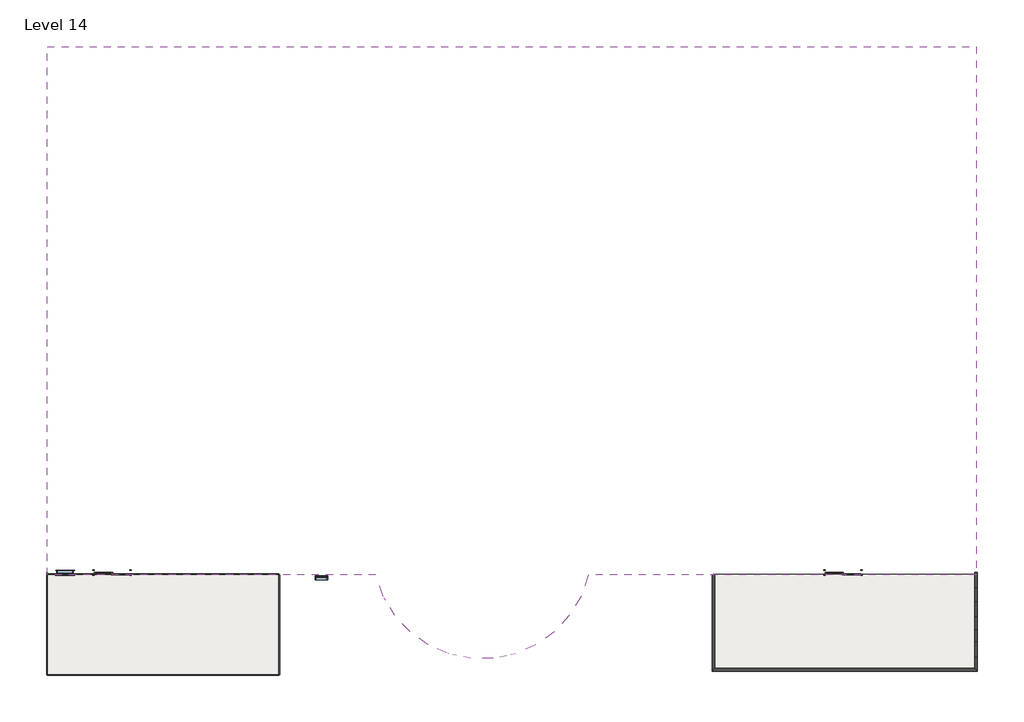
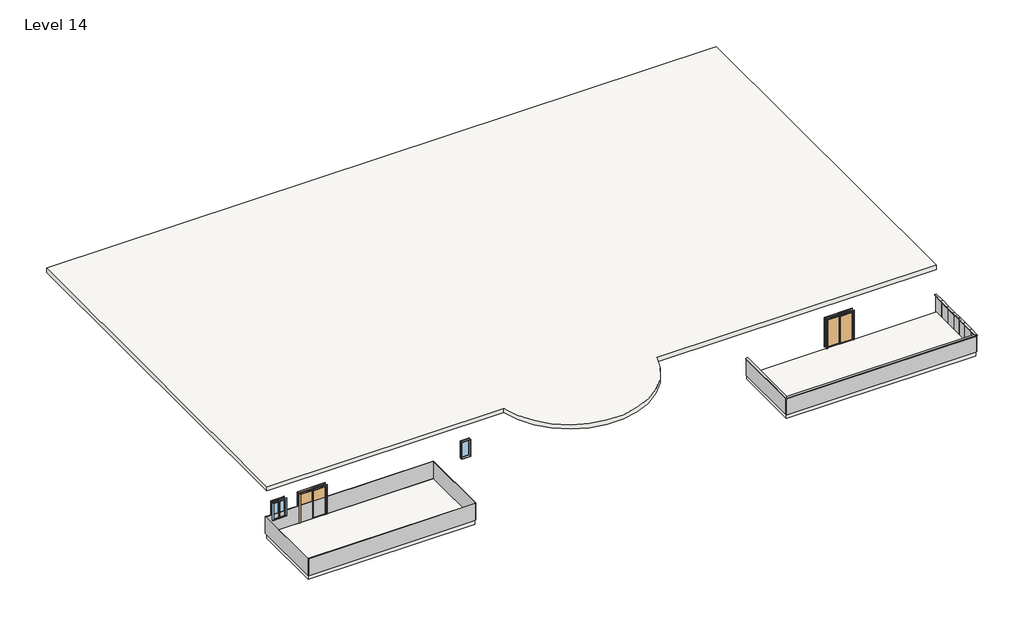
# One storey: 13 plates, 9 members, 3 slabs, 2 doors, 2 windows.
"""IFC4 building model written with IfcOpenShell, lengths in millimetres."""

from ifc_helpers import new_model, si_unit, point, frame, frame_2d, origin, place, context, project, spatial, polyline, circle_curve, trimmed, segment, composite_curve, outline, extrude, transform, mapped, element, save
from components import door_076b30e0, member_47bfaf8a, member_aa870034, member_0b2b3a95, member_df81370e, member_5882a209, member_d818a040, system_panel_glazed_f269d4c8, system_panel_glazed_7af1c9c3, system_panel_glazed_4f3cd66b, system_panel_glazed_7cd9bc56, system_panel_glazed_7fa16c81, system_panel_glazed_ea481271, system_panel_glazed_53c2349a, system_panel_glazed_dfd0d0b7, window_bb17773d, window_80bd9af0

model = new_model("IFC4")

# Units and contexts
model_context = context("Model", 3, world=origin())
ifc_project = project(units=[si_unit("LENGTHUNIT", "METRE", prefix="MILLI")], contexts=[model_context])

# Site, building, storey
site = spatial("IfcSite", under=ifc_project)
building = spatial("IfcBuilding", under=site)
storey = spatial("IfcBuildingStorey", under=building, Name="Level 14", Elevation=23164.8)

# Doors
placement = place(None, origin())
door_shape = door_076b30e0(model_context)
element("IfcDoor", 1, ObjectType="Door-Double-Sliding : 68\" x 80\"", at=placement, inside=storey, context=model_context, shape_type="MappedRepresentation", body=[
    mapped(door_shape, transform((-16674.185279, -12227.7237084, 23164.8), x_axis=(-1.0, 0.0, 0.0), y_axis=(0.0, -1.0, 0.0), z_axis=(0.0, 0.0, 1.0))),
])
element("IfcDoor", 2, ObjectType="Door-Double-Sliding : 68\" x 80\"", at=placement, inside=storey, context=model_context, shape_type="MappedRepresentation", body=[
    mapped(door_shape, transform((18987.414721, -12227.7237084, 23164.8), x_axis=(-1.0, 0.0, 0.0), y_axis=(0.0, -1.0, 0.0), z_axis=(0.0, 0.0, 1.0))),
])

# Members
member_shape = member_47bfaf8a(model_context)
element("IfcMember", 3, ObjectType="Rectangular Mullion : 2.5\" x 5\" rectangular", at=placement, inside=storey, context=model_context, shape_type="MappedRepresentation", body=[
    mapped(member_shape, transform((25489.814721, -15121.4141485, 24384.0), x_axis=(0.0, 0.0, 1.0), y_axis=(-1.0, 0.0, 0.0), z_axis=(0.0, -1.0, 0.0))),
])
element("IfcMember", 4, ObjectType="Rectangular Mullion : 2.5\" x 5\" rectangular", at=placement, inside=storey, context=model_context, shape_type="MappedRepresentation", body=[
    mapped(member_shape, transform((25489.814721, -15731.0141485, 24384.0), x_axis=(0.0, 0.0, 1.0), y_axis=(-1.0, 0.0, 0.0), z_axis=(0.0, -1.0, 0.0))),
])
member_2_shape = member_aa870034(model_context)
element("IfcMember", 5, ObjectType="Rectangular Mullion : 2.5\" x 5\" rectangular", at=placement, inside=storey, context=model_context, shape_type="MappedRepresentation", body=[
    mapped(member_2_shape, transform((25489.814721, -16493.0141485, 24384.0), x_axis=(0.0, 0.0, 1.0), y_axis=(-1.0, 0.0, 0.0), z_axis=(0.0, -1.0, 0.0))),
])
member_3_shape = member_0b2b3a95(model_context)
element("IfcMember", 6, ObjectType="Rectangular Mullion : 2.5\" x 5\" rectangular", at=placement, inside=storey, context=model_context, shape_type="MappedRepresentation", body=[
    mapped(member_3_shape, transform((25489.814721, -13073.7538551, 24384.0), x_axis=(0.0, 0.0, 1.0), y_axis=(-1.0, 0.0, 0.0), z_axis=(0.0, -1.0, 0.0))),
])
element("IfcMember", 7, ObjectType="Rectangular Mullion : 2.5\" x 5\" rectangular", at=placement, inside=storey, context=model_context, shape_type="MappedRepresentation", body=[
    mapped(member_3_shape, transform((25489.814721, -13792.7840018, 24384.0), x_axis=(0.0, 0.0, 1.0), y_axis=(-1.0, 0.0, 0.0), z_axis=(0.0, -1.0, 0.0))),
])
element("IfcMember", 8, ObjectType="Rectangular Mullion : 2.5\" x 5\" rectangular", at=placement, inside=storey, context=model_context, shape_type="MappedRepresentation", body=[
    mapped(member_3_shape, transform((25489.814721, -14511.8141485, 24384.0), x_axis=(0.0, 0.0, 1.0), y_axis=(-1.0, 0.0, 0.0), z_axis=(0.0, -1.0, 0.0))),
])
member_4_shape = member_df81370e(model_context)
element("IfcMember", 9, ObjectType="Rectangular Mullion : 2.5\" x 5\" rectangular", at=placement, inside=storey, context=model_context, shape_type="MappedRepresentation", body=[
    mapped(member_4_shape, transform((25489.814721, -17102.6141485, 24384.0), x_axis=(0.0, 0.0, 1.0), y_axis=(-1.0, 0.0, 0.0), z_axis=(0.0, -1.0, 0.0))),
])
member_5_shape = member_5882a209(model_context)
element("IfcMember", 10, ObjectType="Rectangular Mullion : 2.5\" x 5\" rectangular", at=placement, inside=storey, context=model_context, shape_type="MappedRepresentation", body=[
    mapped(member_5_shape, transform((12667.5594464, -12456.3237084, 24384.0), x_axis=(0.0, 0.0, 1.0), y_axis=(1.0, 0.0, 0.0), z_axis=(0.0, 1.0, 0.0))),
])
member_6_shape = member_d818a040(model_context)
element("IfcMember", 11, ObjectType="Rectangular Mullion : 2.5\" x 5\" rectangular", at=placement, inside=storey, context=model_context, shape_type="MappedRepresentation", body=[
    mapped(member_6_shape, transform((12667.5594464, -17102.6141485, 24384.0), x_axis=(0.0, 0.0, 1.0), y_axis=(0.0, 1.0, 0.0), z_axis=(-1.0, 0.0, 0.0))),
])

# Plates
system_panel_glazed_shape = system_panel_glazed_f269d4c8(model_context)
element("IfcPlate", 12, ObjectType="System Panel : Glazed", at=placement, inside=storey, context=model_context, shape_type="MappedRepresentation", body=[
    mapped(system_panel_glazed_shape, transform((25489.814721, -16112.0141485, 23164.8), x_axis=(0.0, -1.0, 0.0), y_axis=(1.0, 0.0, 0.0), z_axis=(0.0, 0.0, 1.0))),
])
system_panel_glazed_2_shape = system_panel_glazed_7af1c9c3(model_context)
element("IfcPlate", 13, ObjectType="System Panel : Glazed", at=placement, inside=storey, context=model_context, shape_type="MappedRepresentation", body=[
    mapped(system_panel_glazed_2_shape, transform((25489.814721, -16797.8141485, 23164.8), x_axis=(0.0, -1.0, 0.0), y_axis=(1.0, 0.0, 0.0), z_axis=(0.0, 0.0, 1.0))),
])
element("IfcPlate", 14, ObjectType="System Panel : Glazed", at=placement, inside=storey, context=model_context, shape_type="MappedRepresentation", body=[
    mapped(system_panel_glazed_2_shape, transform((25489.814721, -15426.2141485, 23164.8), x_axis=(0.0, -1.0, 0.0), y_axis=(1.0, 0.0, 0.0), z_axis=(0.0, 0.0, 1.0))),
])
element("IfcPlate", 15, ObjectType="System Panel : Glazed", at=placement, inside=storey, context=model_context, shape_type="MappedRepresentation", body=[
    mapped(system_panel_glazed_2_shape, transform((25489.814721, -14816.6141485, 23164.8), x_axis=(0.0, -1.0, 0.0), y_axis=(1.0, 0.0, 0.0), z_axis=(0.0, 0.0, 1.0))),
])
system_panel_glazed_3_shape = system_panel_glazed_4f3cd66b(model_context)
element("IfcPlate", 16, ObjectType="System Panel : Glazed", at=placement, inside=storey, context=model_context, shape_type="MappedRepresentation", body=[
    mapped(system_panel_glazed_3_shape, transform((25489.814721, -12714.2387817, 23164.8), x_axis=(0.0, -1.0, 0.0), y_axis=(1.0, 0.0, 0.0), z_axis=(0.0, 0.0, 1.0))),
])
element("IfcPlate", 17, ObjectType="System Panel : Glazed", at=placement, inside=storey, context=model_context, shape_type="MappedRepresentation", body=[
    mapped(system_panel_glazed_3_shape, transform((25489.814721, -14152.2990751, 23164.8), x_axis=(0.0, -1.0, 0.0), y_axis=(1.0, 0.0, 0.0), z_axis=(0.0, 0.0, 1.0))),
])
element("IfcPlate", 18, ObjectType="System Panel : Glazed", at=placement, inside=storey, context=model_context, shape_type="MappedRepresentation", body=[
    mapped(system_panel_glazed_3_shape, transform((25489.814721, -13433.2689284, 23164.8), x_axis=(0.0, -1.0, 0.0), y_axis=(1.0, 0.0, 0.0), z_axis=(0.0, 0.0, 1.0))),
])
system_panel_glazed_4_shape = system_panel_glazed_7cd9bc56(model_context)
element("IfcPlate", 19, ObjectType="System Panel : Glazed", at=placement, inside=storey, context=model_context, shape_type="MappedRepresentation", body=[
    mapped(system_panel_glazed_4_shape, transform((19078.6870837, -17102.6141485, 23164.8), x_axis=(-1.0, 0.0, 0.0), y_axis=(0.0, -1.0, 0.0), z_axis=(0.0, 0.0, 1.0))),
])
system_panel_glazed_5_shape = system_panel_glazed_7fa16c81(model_context)
element("IfcPlate", 20, ObjectType="System Panel : Glazed", at=placement, inside=storey, context=model_context, shape_type="MappedRepresentation", body=[
    mapped(system_panel_glazed_5_shape, transform((12667.5594464, -14779.4689284, 23164.8), x_axis=(0.0, 1.0, 0.0), y_axis=(-1.0, 0.0, 0.0), z_axis=(0.0, 0.0, 1.0))),
])
system_panel_glazed_6_shape = system_panel_glazed_ea481271(model_context)
element("IfcPlate", 21, ObjectType="System Panel : Glazed", at=placement, inside=storey, context=model_context, shape_type="MappedRepresentation", body=[
    mapped(system_panel_glazed_6_shape, transform((-14184.985279, -12456.3237084, 23164.8), x_axis=(1.0, 0.0, 0.0), y_axis=(0.0, 1.0, 0.0), z_axis=(0.0, 0.0, 1.0))),
])
element("IfcPlate", 22, ObjectType="System Panel : Glazed", at=placement, inside=storey, context=model_context, shape_type="MappedRepresentation", body=[
    mapped(system_panel_glazed_6_shape, transform((-14184.985279, -17333.1237084, 23164.8), x_axis=(-1.0, 0.0, 0.0), y_axis=(0.0, -1.0, 0.0), z_axis=(0.0, 0.0, 1.0))),
])
system_panel_glazed_7_shape = system_panel_glazed_53c2349a(model_context)
element("IfcPlate", 23, ObjectType="System Panel : Glazed", at=placement, inside=storey, context=model_context, shape_type="MappedRepresentation", body=[
    mapped(system_panel_glazed_7_shape, transform((-8546.185279, -14894.7237084, 23164.8), x_axis=(0.0, -1.0, 0.0), y_axis=(1.0, 0.0, 0.0), z_axis=(0.0, 0.0, 1.0))),
])
system_panel_glazed_8_shape = system_panel_glazed_dfd0d0b7(model_context)
element("IfcPlate", 24, ObjectType="System Panel : Glazed", at=placement, inside=storey, context=model_context, shape_type="MappedRepresentation", body=[
    mapped(system_panel_glazed_8_shape, transform((-19823.785279, -14843.9237084, 23164.8), x_axis=(0.0, 1.0, 0.0), y_axis=(-1.0, 0.0, 0.0), z_axis=(0.0, 0.0, 1.0))),
])

# Slabs
element("IfcSlab", 25, ObjectType="Generic - 12\"", at=placement, inside=storey, context=model_context, shape_type="SweptSolid", body=[
    extrude(outline(composite_curve([segment(polyline([(25489.814721, 13330.837176), (25489.814721, -12475.562824), (6571.5594464, -12475.562824)]), True, "CONTINUOUS"), segment(trimmed(circle_curve(frame_2d((1385.214721, -11244.9297828)), 5330.3498284), [point((6571.5594464, -12475.562824))], [point((-3801.1300045, -12475.562824))], False, "CARTESIAN"), True, "CONTINUOUS"), segment(polyline([(-3801.1300045, -12475.562824), (-19823.785279, -12475.562824), (-19823.785279, 13330.837176), (25489.814721, 13330.837176)]), True, "CONTINUOUS")], self_intersect=False)), frame((0.0, 0.0, 26250.5464133), z_axis=(0.0, 0.0, 1.0), x_axis=(1.0, 0.0, 0.0)), (0.0, 0.0, 1.0), 304.8),
])
element("IfcSlab", 26, ObjectType="Generic - 12\"", at=placement, inside=storey, context=model_context, shape_type="SweptSolid", body=[
    extrude(outline(polyline([(25489.814721, -12430.3934399), (25489.814721, -17102.6141485), (12667.5594464, -17102.6141485), (12667.5594464, -12430.3934399), (25489.814721, -12430.3934399)])), frame((0.0, 0.0, 22860.0), z_axis=(0.0, 0.0, 1.0), x_axis=(1.0, 0.0, 0.0)), (0.0, 0.0, 1.0), 304.8),
])
element("IfcSlab", 27, ObjectType="Generic - 12\"", at=placement, inside=storey, context=model_context, shape_type="SweptSolid", body=[
    extrude(outline(polyline([(-8546.185279, -12456.3237084), (-8546.185279, -17333.1237084), (-19823.785279, -17333.1237084), (-19823.785279, -12456.3237084), (-8546.185279, -12456.3237084)])), frame((0.0, 0.0, 22860.0), z_axis=(0.0, 0.0, 1.0), x_axis=(1.0, 0.0, 0.0)), (0.0, 0.0, 1.0), 304.8),
])

# Windows
window_shape = window_bb17773d(model_context)
element("IfcWindow", 28, ObjectType="Casement Dbl with Trim : 32\" x 48\"", at=placement, inside=storey, context=model_context, shape_type="MappedRepresentation", body=[
    mapped(window_shape, transform((-18960.185279, -12335.6737084, 23075.0161382), x_axis=(-1.0, 0.0, 0.0), y_axis=(0.0, -1.0, 0.0), z_axis=(0.0, 0.0, 1.0))),
])
window_2_shape = window_80bd9af0(model_context)
element("IfcWindow", 29, ObjectType="Fixed : 24\" x 48\"", at=placement, inside=storey, context=model_context, shape_type="MappedRepresentation", body=[
    mapped(window_2_shape, transform((-6425.285279, -12617.2007309, 23164.8), x_axis=(1.0, 0.0, 0.0), y_axis=(0.0, 1.0, 0.0), z_axis=(0.0, 0.0, 1.0))),
])

save(model, "model.ifc")

# Revit data of these elements
# Type "Door-Double-Sliding : 68\" x 80\""
#   Type Mark = "10"
#   Construction Type Id = "opn-d45"
#   Assembly Code = "C1020"
#   Analytic Construction = "Wood frame, double glass door "
#   Thickness = 0' - 2"
#   Thermal Resistance (R) = 1.8150 (h·ft²·°F)/BTU
#   Heat Transfer Coefficient (U) = 0.5510 BTU/(h·ft²·°F)
#   Height = 6' - 8"
#   Rail Width = 0' - 2"
#   Stiles = 0' - 2"
#   Trim Projection Ext = 0' - 1"
#   Trim Projection Int = 0' - 1"
#   Trim Width = 0' - 3"
#   Width = 5' - 8"
#   Define Thermal Properties by = 1
#   Glazing = Glass
#   Panel Material = Wood - Birch - Solid Stained Light Low Gloss
#   Trim Material = Paint - Sienna
#   Visual Light Transmittance = 0
#   Solar Heat Gain Coefficient = 0
#   Function = (empty or 0)
#   Wall Closure = (empty or 0)
# Type "Rectangular Mullion : 2.5\" x 5\" rectangular"
#   built-in parameter 1007304 = 0.416667 (stored number, unit not read)
#   built-in parameter 1007301 = 0.104167 (stored number, unit not read)
#   built-in parameter 1007300 = 0.104167 (stored number, unit not read)
# Type "System Panel : Glazed"
#   Construction Type Id = "GSP4R"
#   Analytic Construction = "1/8 in Pilkington single glazing"
#   Visual Light Transmittance = 0.9
#   Solar Heat Gain Coefficient = 0.86
#   Heat Transfer Coefficient (U) = 1.18115 BTU/(h·ft²·°F)
# Type "Generic - 12\""
#   Assembly Code = "B1010"
#   Function = 0
#   Layers, outside or top first: 1' - 0" no material (function 1)
# Type "Casement Dbl with Trim : 32\" x 48\""
#   Type Mark = "36"
#   Construction Type Id = "GSP4R"
#   Assembly Code = "B2020100"
#   Analytic Construction = "1/8 in Pilkington single glazing"
#   Visual Light Transmittance = 0.9
#   Solar Heat Gain Coefficient = 0.78
#   Heat Transfer Coefficient (U) = 0.6496 BTU/(h·ft²·°F)
#   Height = 4' - 0"
#   Default Sill Height = 3' - 0"
#   Trim Projection - Ext. = 0' - 0 1/2"
#   Trim Projection - Int. = 0' - 0 3/4"
#   Trim Width - Exterior = 0' - 3 1/2"
#   Trim Width - Interior = 0' - 3 1/2"
#   Width = 2' - 8"
#   Window Inset = 0' - 0 3/4"
#   Define Thermal Properties by = 1
#   Glass Pane Material = Glass
#   Sash Material = Sash
#   Trim Exterior Material = Trim
#   Trim Interior Material = Trim
#   Wall Closure = (empty or 0)
# Type "Fixed : 24\" x 48\""
#   Type Mark = "2"
#   Construction Type Id = "GSP4R"
#   Assembly Code = "B2020100"
#   Analytic Construction = "1/8 in Pilkington single glazing"
#   Visual Light Transmittance = 0.9
#   Solar Heat Gain Coefficient = 0.78
#   Heat Transfer Coefficient (U) = 0.6496 BTU/(h·ft²·°F)
#   Height = 4' - 0"
#   Default Sill Height = 3' - 0"
#   Width = 2' - 0"
#   Window Inset = 0' - 0 3/4"
#   Define Thermal Properties by = 1
#   Glass Pane Material = Glass
#   Sash Material = Sash
#   Wall Closure = (empty or 0)
# Elements 1, 2 (IfcDoor, "Door-Double-Sliding : 68\" x 80\"")
#   Phase Created = New Construction
#   Materials on its faces: "Paint - Sienna", "Wood - Birch - Solid Stained Light Low Gloss", "Glass"
# Elements 3, 4, 5, 6, 7, 8, 9, 10, 11 (IfcMember, "Rectangular Mullion : 2.5\" x 5\" rectangular")
#   Phase Created = New Construction
#   Materials on its faces: "Aluminum"
# Elements 12, 13, 14, 15, 16, 17, 18, 19, 20, 21, 22, 23, 24 (IfcPlate, "System Panel : Glazed")
#   Phase Created = New Construction
#   Materials on its faces: "Glass"
# Element 25 (IfcSlab, "Generic - 12\"")
#   Height Offset From Level = 11' - 1.48608"
#   Phase Created = New Construction
#   Materials on its faces: "Default Floor"
# Elements 26, 27 (IfcSlab, "Generic - 12\"")
#   Height Offset From Level = 0' - 0"
#   Phase Created = New Construction
#   Materials on its faces: "Default Floor"
# Element 28 (IfcWindow, "Casement Dbl with Trim : 32\" x 48\"")
#   Mark = "44"
#   Phase Created = New Construction
#   Materials on its faces: "Sash", "Trim", "Glass"
# Element 29 (IfcWindow, "Fixed : 24\" x 48\"")
#   Mark = "78"
#   Phase Created = New Construction
#   Materials on its faces: "Sash", "Glass"
# Materials
#   "Glass": class "Glass", colour RGB 0 128 192, transparency 0.75, Description = "Soda Lime Glass", Cost = 0
#   "Wood - Birch - Solid Stained Light Low Gloss": class "Wood", colour RGB 210 159 95, transparency 0, Cost = 0
#   "Paint - Sienna": colour RGB 118 70 51, transparency 0, Cost = 0
#   "Sash": class "Wood", colour RGB 224 178 126, transparency 0
#   "Trim": class "Wood", colour RGB 224 178 126, transparency 0
#   "Aluminum": class "Metal", colour RGB 247 247 247, transparency 0, Description = "Aluminum 6061", Cost = 0
#   "Default Floor": colour RGB 128 128 128, transparency 0
